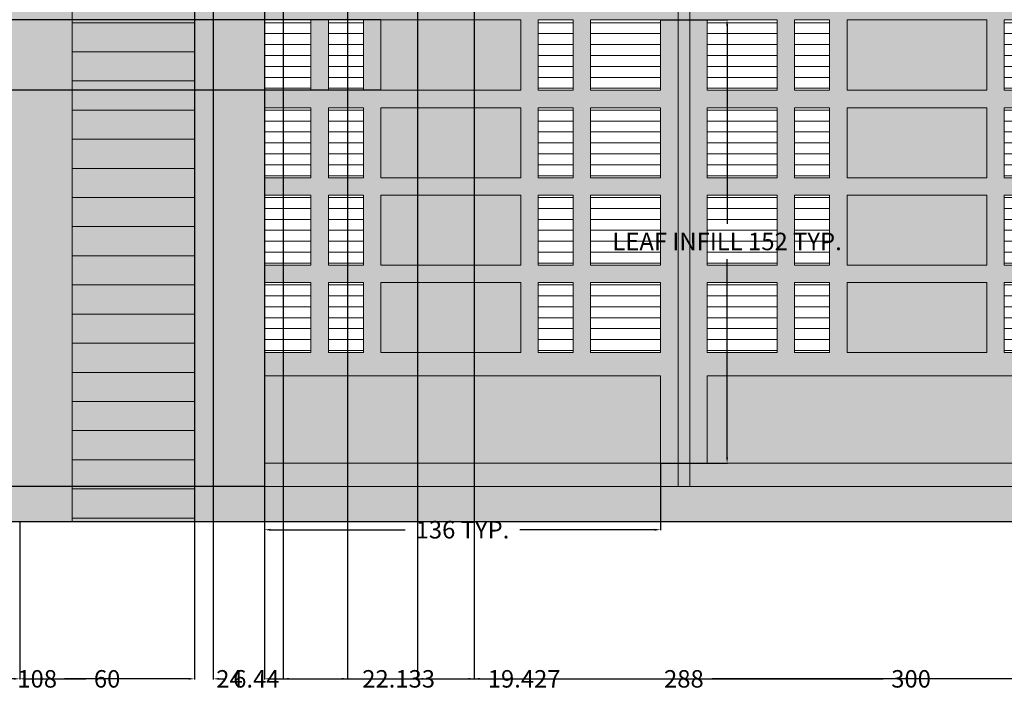
# Model space of a CAD drawing. Units: inches. Extents: x 180 to 1069, y 71 to 1267.
# Tile 2 of 8: x 546 to 884, y 71 to 301. Entities that reach past the tile are written whole.
import ezdxf

# ---------------------------------------------------------------- set-up
doc = ezdxf.new("R2010")
doc.units = ezdxf.units.IN
doc.header["$MEASUREMENT"] = 0
for name, color, linetype, lineweight in [('A-ANNO-DIMS', 2, 'Continuous', 18), ('A-COLS', 7, 'Continuous', 25), ('A-DOOR-GATE', 7, 'Continuous', 18), ('A-DOOR-PANL-PATT', 25, 'Continuous', 13), ('A-WALL', 7, 'Continuous', 30), ('A-WALL-CLAD', 7, 'Continuous', 18), ('A-WALL-CLAD-JNTS-PATT', 18, 'Continuous', 13), ('A-WALL-CLAD-PATT', 26, 'Continuous', 13)]:
    doc.layers.add(name, color=color, linetype=linetype, lineweight=lineweight)
for name, color, linetype, lineweight, true_color in [('A-DOOR-GATE-PATT', 18, 'Continuous', 13, 0x000000), ('A-DOOR-HARD-PATT', 8, 'Continuous', 13, 0x7f7f6c), ('A-DOOR-SHUT-PATT', 254, 'Continuous', 13, 0xb7d9eb), ('A-ELEV-FRAM-PATT', 53, 'Continuous', 13, 0xefd648)]:
    doc.layers.add(name, color=color, linetype=linetype, lineweight=lineweight, true_color=true_color)
doc.styles.get("Standard").update_dxf_attribs({"font": 'arial.ttf'})
doc.dimstyles.get("Standard").update_dxf_attribs({"dimtxt": 6, "dimasz": 2, "dimexe": 0.18, "dimexo": 0.0625, "dimgap": 3, "dimtad": 0, "dimtih": 1, "dimtoh": 1, "dimdec": 0, "dimzin": 0, "dimdsep": 46, "dimlunit": 3, "dimtxsty": 'Standard', "dimcen": 0.09, "dimadec": 0, "dimazin": 0, "dimtfac": 1, "dimtdec": 0, "dimtofl": 0, "dimtmove": 0, "dimatfit": 3, "dimfxl": 1, "dimtolj": 1, "dimtzin": 0, "dimarcsym": 0})

# ---------------------------------------------------------------- blocks, each defined once
blk = doc.blocks.new('GATE-LEAF-LOWER-INFILL')
for p, q in [((0, 152.23), (16, 152.23)), ((16, 152.23), (16, 128)), ((22, 152.23), (34, 152.23)), ((22, 152.23), (22, 128)), ((34, 152.23), (34, 128)), ((40, 152.23), (88, 152.23)), ((40, 152.23), (40, 128)), ((88, 152.23), (88, 128)), ((94, 152.23), (106, 152.23)), ((94, 152.23), (94, 128)), ((106, 152.23), (106, 128)), ((112, 152.23), (136, 152.23)), ((112, 152.23), (112, 128)), ((136, 152.23), (136, 128)), ((0, 128), (16, 128)), ((22, 128), (34, 128)), ((40, 128), (88, 128)), ((94, 128), (106, 128)), ((112, 128), (136, 128)), ((0, 122), (16, 122)), ((16, 122), (16, 98)), ((22, 122), (34, 122)), ((22, 122), (22, 98)), ((34, 122), (34, 98)), ((40, 122), (88, 122)), ((40, 122), (40, 98)), ((88, 122), (88, 98)), ((94, 122), (106, 122)), ((94, 122), (94, 98)), ((106, 122), (106, 98)), ((112, 122), (136, 122)), ((112, 122), (112, 98)), ((136, 122), (136, 98)), ((0, 98), (16, 98)), ((22, 98), (34, 98)), ((40, 98), (88, 98)), ((94, 98), (106, 98)), ((112, 98), (136, 98)), ((0, 92), (16, 92)), ((16, 92), (16, 68)), ((22, 92), (34, 92)), ((22, 92), (22, 68)), ((34, 92), (34, 68)), ((40, 92), (88, 92)), ((40, 92), (40, 68)), ((88, 92), (88, 68)), ((94, 92), (106, 92)), ((94, 92), (94, 68)), ((106, 92), (106, 68)), ((112, 92), (136, 92)), ((112, 92), (112, 68)), ((136, 92), (136, 68)), ((0, 68), (16, 68)), ((22, 68), (34, 68)), ((40, 68), (88, 68)), ((94, 68), (106, 68)), ((112, 68), (136, 68)), ((0, 62), (16, 62)), ((16, 62), (16, 38)), ((22, 62), (34, 62)), ((22, 62), (22, 38)), ((34, 62), (34, 38)), ((40, 62), (88, 62)), ((40, 62), (40, 38)), ((88, 62), (88, 38)), ((94, 62), (106, 62)), ((94, 62), (94, 38)), ((106, 62), (106, 38)), ((112, 62), (136, 62)), ((112, 62), (112, 38)), ((136, 62), (136, 38)), ((0, 38), (16, 38)), ((22, 38), (34, 38)), ((40, 38), (88, 38)), ((94, 38), (106, 38)), ((112, 38), (136, 38)), ((0, 30), (136, 30)), ((136, 30), (136, 0)), ((0, 0), (136, 0))]:
    blk.add_line(p, q)
blk = doc.blocks.new('*D14')
at = {"layer": 'A-ANNO-DIMS', "color": 0, "lineweight": -2, "transparency": 16777216}
for p, q in [((766.15, 301.05), (789.1, 301.05)), ((788.92, 299.05), (788.92, 231)), ((788.92, 150.82), (788.92, 218.87)), ((766.15, 148.82), (789.1, 148.82))]:
    blk.add_line(p, q, dxfattribs=at)
at = {"layer": 'A-ANNO-DIMS', "color": 0, "transparency": 16777216}
for points in [[(788.59, 299.05), (789.26, 299.05), (788.92, 301.05)], [(788.59, 150.82), (789.26, 150.82), (788.92, 148.82)]]:
    blk.add_solid(points, dxfattribs=at)
at = {"layer": 'Defpoints', "color": 0, "transparency": 16777216}
for p in [(766.09, 301.05), (788.92, 301.05), (766.09, 148.82)]:
    blk.add_point(p, dxfattribs=at)
at = {"layer": 'A-ANNO-DIMS', "color": 0, "transparency": 16777216, "insert": (788.92, 224.93), "char_height": 6, "attachment_point": 5}
blk.add_mtext('\\A1;LEAF INFILL 152 TYP.', dxfattribs=at)
blk = doc.blocks.new('*D15')
at = {"layer": 'A-ANNO-DIMS', "color": 0, "lineweight": -2, "transparency": 16777216}
for p, q in [((630.09, 148.75), (630.09, 125.8)), ((766.09, 148.75), (766.09, 125.8)), ((632.09, 125.98), (678.44, 125.98)), ((764.09, 125.98), (717.74, 125.98))]:
    blk.add_line(p, q, dxfattribs=at)
at = {"layer": 'A-ANNO-DIMS', "color": 0, "transparency": 16777216}
for points in [[(632.09, 126.31), (632.09, 125.65), (630.09, 125.98)], [(764.09, 126.31), (764.09, 125.65), (766.09, 125.98)]]:
    blk.add_solid(points, dxfattribs=at)
at = {"layer": 'Defpoints', "color": 0, "transparency": 16777216}
for p in [(630.09, 148.82), (766.09, 148.82), (766.09, 125.98)]:
    blk.add_point(p, dxfattribs=at)
at = {"layer": 'A-ANNO-DIMS', "color": 0, "transparency": 16777216, "insert": (698.09, 125.98), "char_height": 6, "attachment_point": 5}
blk.add_mtext('\\A1;136 TYP.', dxfattribs=at)
blk = doc.blocks.new('*D29')
at = {"layer": 'A-ANNO-DIMS', "color": 0, "lineweight": -2, "transparency": 16777216}
for p, q in [((306.09, 128.75), (306.09, 74.62)), ((546.09, 128.75), (546.09, 74.62)), ((308.09, 74.8), (416.42, 74.8)), ((544.09, 74.8), (435.76, 74.8))]:
    blk.add_line(p, q, dxfattribs=at)
at = {"layer": 'A-ANNO-DIMS', "color": 0, "transparency": 16777216}
for points in [[(308.09, 75.14), (308.09, 74.47), (306.09, 74.8)], [(544.09, 75.14), (544.09, 74.47), (546.09, 74.8)]]:
    blk.add_solid(points, dxfattribs=at)
at = {"layer": 'Defpoints', "color": 0, "transparency": 16777216}
for p in [(306.09, 128.82), (546.09, 128.82), (546.09, 74.8)]:
    blk.add_point(p, dxfattribs=at)
at = {"layer": 'A-ANNO-DIMS', "color": 0, "transparency": 16777216, "insert": (426.09, 74.8), "char_height": 6, "attachment_point": 5}
blk.add_mtext('\\A1;240', dxfattribs=at)
blk = doc.blocks.new('*D30')
at = {"layer": 'A-ANNO-DIMS', "color": 0, "lineweight": -2, "transparency": 16777216}
for p, q in [((546.09, 128.75), (546.09, 74.62)), ((606.09, 128.75), (606.09, 74.62)), ((548.09, 74.8), (568.78, 74.8)), ((604.09, 74.8), (583.39, 74.8))]:
    blk.add_line(p, q, dxfattribs=at)
at = {"layer": 'A-ANNO-DIMS', "color": 0, "transparency": 16777216}
for points in [[(548.09, 75.14), (548.09, 74.47), (546.09, 74.8)], [(604.09, 75.14), (604.09, 74.47), (606.09, 74.8)]]:
    blk.add_solid(points, dxfattribs=at)
at = {"layer": 'Defpoints', "color": 0, "transparency": 16777216}
for p in [(546.09, 128.82), (606.09, 128.82), (606.09, 74.8)]:
    blk.add_point(p, dxfattribs=at)
at = {"layer": 'A-ANNO-DIMS', "color": 0, "transparency": 16777216, "insert": (576.09, 74.8), "char_height": 6, "attachment_point": 5}
blk.add_mtext('\\A1;60', dxfattribs=at)
blk = doc.blocks.new('*D31')
at = {"layer": 'A-ANNO-DIMS', "color": 0, "lineweight": -2, "transparency": 16777216}
for p, q in [((546.15, 416.82), (1056.28, 416.82)), ((1056.1, 414.82), (1056.1, 278.88)), ((1056.1, 130.82), (1056.1, 266.75)), ((546.15, 128.82), (1056.28, 128.82))]:
    blk.add_line(p, q, dxfattribs=at)
at = {"layer": 'A-ANNO-DIMS', "color": 0, "transparency": 16777216}
for points in [[(1055.77, 414.82), (1056.43, 414.82), (1056.1, 416.82)], [(1055.77, 130.82), (1056.43, 130.82), (1056.1, 128.82)]]:
    blk.add_solid(points, dxfattribs=at)
at = {"layer": 'Defpoints', "color": 0, "transparency": 16777216}
for p in [(546.09, 416.82), (1056.1, 416.82), (546.09, 128.82)]:
    blk.add_point(p, dxfattribs=at)
at = {"layer": 'A-ANNO-DIMS', "color": 0, "transparency": 16777216, "insert": (1056.1, 272.82), "char_height": 6, "attachment_point": 5}
blk.add_mtext('\\A1;288', dxfattribs=at)
blk = doc.blocks.new('*D33')
at = {"layer": 'A-ANNO-DIMS', "color": 0, "lineweight": -2, "transparency": 16777216}
for p, q in [((606.09, 128.75), (606.09, 74.62)), ((630.09, 128.75), (630.09, 74.62)), ((604.09, 74.8), (602.09, 74.8)), ((632.09, 74.8), (634.09, 74.8))]:
    blk.add_line(p, q, dxfattribs=at)
at = {"layer": 'A-ANNO-DIMS', "color": 0, "transparency": 16777216}
for points in [[(604.09, 75.14), (604.09, 74.47), (606.09, 74.8)], [(632.09, 75.14), (632.09, 74.47), (630.09, 74.8)]]:
    blk.add_solid(points, dxfattribs=at)
at = {"layer": 'Defpoints', "color": 0, "transparency": 16777216}
for p in [(606.09, 128.82), (630.09, 128.82), (630.09, 74.8)]:
    blk.add_point(p, dxfattribs=at)
at = {"layer": 'A-ANNO-DIMS', "color": 0, "transparency": 16777216, "insert": (618.09, 74.8), "char_height": 6, "attachment_point": 5}
blk.add_mtext('\\A1;24', dxfattribs=at)
blk = doc.blocks.new('*D34')
at = {"layer": 'A-ANNO-DIMS', "color": 0, "lineweight": -2, "transparency": 16777216}
for p, q in [((630.09, 128.75), (630.09, 74.62)), ((918.09, 128.75), (918.09, 74.62)), ((632.09, 74.8), (764.4, 74.8)), ((916.09, 74.8), (783.77, 74.8))]:
    blk.add_line(p, q, dxfattribs=at)
at = {"layer": 'A-ANNO-DIMS', "color": 0, "transparency": 16777216}
for points in [[(632.09, 75.14), (632.09, 74.47), (630.09, 74.8)], [(916.09, 75.14), (916.09, 74.47), (918.09, 74.8)]]:
    blk.add_solid(points, dxfattribs=at)
at = {"layer": 'Defpoints', "color": 0, "transparency": 16777216}
for p in [(630.09, 128.82), (918.09, 128.82), (918.09, 74.8)]:
    blk.add_point(p, dxfattribs=at)
at = {"layer": 'A-ANNO-DIMS', "color": 0, "transparency": 16777216, "insert": (774.09, 74.8), "char_height": 6, "attachment_point": 5}
blk.add_mtext('\\A1;288', dxfattribs=at)
blk = doc.blocks.new('*D39')
at = {"layer": 'A-ANNO-DIMS', "color": 0, "lineweight": -2, "transparency": 16777216}
for p, q in [((630.02, 346.05), (191.89, 346.05)), ((192.07, 344.05), (192.07, 249.5)), ((192.07, 142.82), (192.07, 237.37)), ((630.02, 140.82), (191.89, 140.82))]:
    blk.add_line(p, q, dxfattribs=at)
at = {"layer": 'A-ANNO-DIMS', "color": 0, "transparency": 16777216}
for points in [[(191.74, 344.05), (192.41, 344.05), (192.07, 346.05)], [(191.74, 142.82), (192.41, 142.82), (192.07, 140.82)]]:
    blk.add_solid(points, dxfattribs=at)
at = {"layer": 'Defpoints', "color": 0, "transparency": 16777216}
for p in [(192.07, 346.05), (630.09, 346.05), (630.09, 140.82)]:
    blk.add_point(p, dxfattribs=at)
at = {"layer": 'A-ANNO-DIMS', "color": 0, "transparency": 16777216, "insert": (192.07, 243.43), "char_height": 6, "attachment_point": 5}
blk.add_mtext('\\A1;205.23', dxfattribs=at)
blk = doc.blocks.new('*D43')
at = {"layer": 'A-ANNO-DIMS', "color": 0, "lineweight": -2, "transparency": 16777216}
for p, q in [((670.02, 301.05), (191.89, 301.05)), ((192.07, 299.05), (192.07, 295)), ((192.07, 278.82), (192.07, 282.87)), ((670.02, 276.82), (191.89, 276.82))]:
    blk.add_line(p, q, dxfattribs=at)
at = {"layer": 'A-ANNO-DIMS', "color": 0, "transparency": 16777216}
for points in [[(191.74, 299.05), (192.41, 299.05), (192.07, 301.05)], [(191.74, 278.82), (192.41, 278.82), (192.07, 276.82)]]:
    blk.add_solid(points, dxfattribs=at)
at = {"layer": 'Defpoints', "color": 0, "transparency": 16777216}
for p in [(670.09, 301.05), (192.07, 276.82), (670.09, 276.82)]:
    blk.add_point(p, dxfattribs=at)
at = {"layer": 'A-ANNO-DIMS', "color": 0, "transparency": 16777216, "insert": (192.07, 288.93), "char_height": 6, "attachment_point": 5}
blk.add_mtext('\\A1;24.23', dxfattribs=at)
blk = doc.blocks.new('*D58')
at = {"layer": 'A-ANNO-DIMS', "color": 0, "lineweight": -2, "transparency": 16777216}
for p, q in [((606.09, 1010.75), (606.09, 74.62)), ((498.09, 956.75), (498.09, 74.62)), ((500.09, 74.8), (542.74, 74.8)), ((604.09, 74.8), (561.44, 74.8))]:
    blk.add_line(p, q, dxfattribs=at)
at = {"layer": 'A-ANNO-DIMS', "color": 0, "transparency": 16777216}
for points in [[(500.09, 75.14), (500.09, 74.47), (498.09, 74.8)], [(604.09, 75.14), (604.09, 74.47), (606.09, 74.8)]]:
    blk.add_solid(points, dxfattribs=at)
at = {"layer": 'Defpoints', "color": 0, "transparency": 16777216}
for p in [(606.09, 1010.82), (498.09, 956.82), (606.09, 74.8)]:
    blk.add_point(p, dxfattribs=at)
at = {"layer": 'A-ANNO-DIMS', "color": 0, "transparency": 16777216, "insert": (552.09, 74.8), "char_height": 6, "attachment_point": 5}
blk.add_mtext('\\A1;108', dxfattribs=at)
blk = doc.blocks.new('*D65')
at = {"layer": 'A-ANNO-DIMS', "color": 0, "lineweight": -2, "transparency": 16777216}
for p, q in [((636.53, 557.75), (636.53, 74.62)), ((658.66, 557.75), (658.66, 74.62)), ((638.53, 74.8), (656.66, 74.8)), ((658.66, 74.8), (660.66, 74.8))]:
    blk.add_line(p, q, dxfattribs=at)
at = {"layer": 'A-ANNO-DIMS', "color": 0, "transparency": 16777216}
for points in [[(638.53, 75.14), (638.53, 74.47), (636.53, 74.8)], [(656.66, 75.14), (656.66, 74.47), (658.66, 74.8)]]:
    blk.add_solid(points, dxfattribs=at)
at = {"layer": 'Defpoints', "color": 0, "transparency": 16777216}
for p in [(636.53, 557.82), (658.66, 557.82), (658.66, 74.8)]:
    blk.add_point(p, dxfattribs=at)
at = {"layer": 'A-ANNO-DIMS', "color": 0, "transparency": 16777216, "insert": (676.17, 74.8), "char_height": 6, "attachment_point": 5}
blk.add_mtext('\\A1;22.133', dxfattribs=at)
blk = doc.blocks.new('*D66')
at = {"layer": 'A-ANNO-DIMS', "color": 0, "lineweight": -2, "transparency": 16777216}
for p, q in [((606.09, 647.75), (606.09, 74.62)), ((612.53, 557.75), (612.53, 74.62)), ((604.09, 74.8), (602.09, 74.8)), ((614.53, 74.8), (616.53, 74.8))]:
    blk.add_line(p, q, dxfattribs=at)
at = {"layer": 'A-ANNO-DIMS', "color": 0, "transparency": 16777216}
for points in [[(604.09, 75.14), (604.09, 74.47), (606.09, 74.8)], [(614.53, 75.14), (614.53, 74.47), (612.53, 74.8)]]:
    blk.add_solid(points, dxfattribs=at)
at = {"layer": 'Defpoints', "color": 0, "transparency": 16777216}
for p in [(606.09, 647.82), (612.53, 557.82), (612.53, 74.8)]:
    blk.add_point(p, dxfattribs=at)
at = {"layer": 'A-ANNO-DIMS', "color": 0, "transparency": 16777216, "insert": (627.32, 74.8), "char_height": 6, "attachment_point": 5}
blk.add_mtext('\\A1;6.44', dxfattribs=at)
blk = doc.blocks.new('*D67')
at = {"layer": 'A-ANNO-DIMS', "color": 0, "lineweight": -2, "transparency": 16777216}
for p, q in [((682.66, 557.75), (682.66, 74.62)), ((702.09, 557.75), (702.09, 74.62)), ((684.66, 74.8), (700.09, 74.8)), ((702.09, 74.8), (704.09, 74.8))]:
    blk.add_line(p, q, dxfattribs=at)
at = {"layer": 'A-ANNO-DIMS', "color": 0, "transparency": 16777216}
for points in [[(684.66, 75.14), (684.66, 74.47), (682.66, 74.8)], [(700.09, 75.14), (700.09, 74.47), (702.09, 74.8)]]:
    blk.add_solid(points, dxfattribs=at)
at = {"layer": 'Defpoints', "color": 0, "transparency": 16777216}
for p in [(682.66, 557.82), (702.09, 557.82), (702.09, 74.8)]:
    blk.add_point(p, dxfattribs=at)
at = {"layer": 'A-ANNO-DIMS', "color": 0, "transparency": 16777216, "insert": (719.26, 74.8), "char_height": 6, "attachment_point": 5}
blk.add_mtext('\\A1;19.427', dxfattribs=at)
blk = doc.blocks.new('*D68')
at = {"layer": 'A-ANNO-DIMS', "color": 0, "lineweight": -2, "transparency": 16777216}
for p, q in [((702.09, 557.75), (702.09, 74.62)), ((1002.09, 557.75), (1002.09, 74.62)), ((704.09, 74.8), (842.47, 74.8)), ((1000.09, 74.8), (861.7, 74.8))]:
    blk.add_line(p, q, dxfattribs=at)
at = {"layer": 'A-ANNO-DIMS', "color": 0, "transparency": 16777216}
for points in [[(704.09, 75.14), (704.09, 74.47), (702.09, 74.8)], [(1000.09, 75.14), (1000.09, 74.47), (1002.09, 74.8)]]:
    blk.add_solid(points, dxfattribs=at)
at = {"layer": 'Defpoints', "color": 0, "transparency": 16777216}
for p in [(702.09, 557.82), (1002.09, 557.82), (1002.09, 74.8)]:
    blk.add_point(p, dxfattribs=at)
at = {"layer": 'A-ANNO-DIMS', "color": 0, "transparency": 16777216, "insert": (852.09, 74.8), "char_height": 6, "attachment_point": 5}
blk.add_mtext('\\A1;300', dxfattribs=at)

msp = doc.modelspace()

# ---------------------------------------------------------------- hatches: boundary and pattern name
at = {"layer": 'A-DOOR-GATE-PATT'}
h = msp.add_hatch(color=256, dxfattribs=at)
h.dxf.hatch_style = 1
h.paths.add_polyline_path([(772.0875, 346.0477), (630.0875, 346.0477), (630.0875, 338.0477), (646.0875, 338.0477), (646.0875, 307.0477), (630.0875, 307.0477), (630.0875, 301.0477), (646.0875, 301.0477), (646.0875, 276.8159), (630.0875, 276.8159), (630.0875, 270.8159), (646.0875, 270.8159), (646.0875, 246.8159), (630.0875, 246.8159), (630.0875, 240.8159), (646.0875, 240.8159), (646.0875, 216.8159), (630.0875, 216.8159), (630.0875, 210.8159), (646.0875, 210.8159), (646.0875, 186.8159), (630.0875, 186.8159), (630.0875, 178.8159), (766.0875, 178.8159), (766.0875, 148.8159), (630.0875, 148.8159), (630.0875, 140.8159), (772.0875, 140.8159)])
h.paths.add_polyline_path([(670.0875, 338.0477), (718.0875, 338.0477), (718.0875, 307.0477), (670.0875, 307.0477)], flags=16)
h.paths.add_polyline_path([(664.0875, 338.0477), (664.0875, 307.0477), (652.0875, 307.0477), (652.0875, 338.0477)], flags=16)
h.paths.add_polyline_path([(670.0875, 301.0477), (718.0875, 301.0477), (718.0875, 276.8159), (670.0875, 276.8159)], flags=16)
h.paths.add_polyline_path([(664.0875, 301.0477), (664.0875, 276.8159), (652.0875, 276.8159), (652.0875, 301.0477)], flags=16)
h.paths.add_polyline_path([(724.0875, 338.0477), (736.0875, 338.0477), (736.0875, 307.0477), (724.0875, 307.0477)], flags=16)
h.paths.add_polyline_path([(724.0875, 301.0477), (736.0875, 301.0477), (736.0875, 276.8159), (724.0875, 276.8159)], flags=16)
h.paths.add_polyline_path([(670.0875, 270.8159), (718.0875, 270.8159), (718.0875, 246.8159), (670.0875, 246.8159)], flags=16)
h.paths.add_polyline_path([(664.0875, 270.8159), (664.0875, 246.8159), (652.0875, 246.8159), (652.0875, 270.8159)], flags=16)
h.paths.add_polyline_path([(742.0875, 338.0477), (766.0875, 338.0477), (766.0875, 307.0477), (742.0875, 307.0477)], flags=16)
h.paths.add_polyline_path([(742.0875, 301.0477), (766.0875, 301.0477), (766.0875, 276.8159), (742.0875, 276.8159)], flags=16)
h.paths.add_polyline_path([(724.0875, 270.8159), (736.0875, 270.8159), (736.0875, 246.8159), (724.0875, 246.8159)], flags=16)
h.paths.add_polyline_path([(670.0875, 240.8159), (718.0875, 240.8159), (718.0875, 216.8159), (670.0875, 216.8159)], flags=16)
h.paths.add_polyline_path([(664.0875, 240.8159), (664.0875, 216.8159), (652.0875, 216.8159), (652.0875, 240.8159)], flags=16)
h.paths.add_polyline_path([(742.0875, 270.8159), (766.0875, 270.8159), (766.0875, 246.8159), (742.0875, 246.8159)], flags=16)
h.paths.add_polyline_path([(724.0875, 240.8159), (736.0875, 240.8159), (736.0875, 216.8159), (724.0875, 216.8159)], flags=16)
h.paths.add_polyline_path([(742.0875, 240.8159), (766.0875, 240.8159), (766.0875, 216.8159), (742.0875, 216.8159)], flags=16)
h.paths.add_polyline_path([(670.0875, 210.8159), (718.0875, 210.8159), (718.0875, 186.8159), (670.0875, 186.8159)], flags=16)
h.paths.add_polyline_path([(664.0875, 210.8159), (664.0875, 186.8159), (652.0875, 186.8159), (652.0875, 210.8159)], flags=16)
h.paths.add_polyline_path([(724.0875, 210.8159), (736.0875, 210.8159), (736.0875, 186.8159), (724.0875, 186.8159)], flags=16)
h.paths.add_polyline_path([(742.0875, 210.8159), (766.0875, 210.8159), (766.0875, 186.8159), (742.0875, 186.8159)], flags=16)
h.paths.add_polyline_path([(918.0875, 346.0477), (776.0875, 346.0477), (776.0875, 140.8159), (918.0875, 140.8159), (918.0875, 148.8159), (782.0875, 148.8159), (782.0875, 178.8159), (918.0875, 178.8159), (918.0875, 186.8159), (902.0875, 186.8159), (902.0875, 210.8159), (918.0875, 210.8159), (918.0875, 216.8159), (902.0875, 216.8159), (902.0875, 240.8159), (918.0875, 240.8159), (918.0875, 246.8159), (902.0875, 246.8159), (902.0875, 270.8159), (918.0875, 270.8159), (918.0875, 276.8159), (902.0875, 276.8159), (902.0875, 301.0477), (918.0875, 301.0477), (918.0875, 307.0477), (902.0875, 307.0477), (902.0875, 338.0477), (918.0875, 338.0477)])
h.paths.add_polyline_path([(782.0875, 338.0477), (806.0875, 338.0477), (806.0875, 307.0477), (782.0875, 307.0477)], flags=16)
h.paths.add_polyline_path([(812.0875, 338.0477), (824.0875, 338.0477), (824.0875, 307.0477), (812.0875, 307.0477)], flags=16)
h.paths.add_polyline_path([(782.0875, 301.0477), (806.0875, 301.0477), (806.0875, 276.8159), (782.0875, 276.8159)], flags=16)
h.paths.add_polyline_path([(830.0875, 338.0477), (878.0875, 338.0477), (878.0875, 307.0477), (830.0875, 307.0477)], flags=16)
h.paths.add_polyline_path([(812.0875, 301.0477), (824.0875, 301.0477), (824.0875, 276.8159), (812.0875, 276.8159)], flags=16)
h.paths.add_polyline_path([(830.0875, 301.0477), (878.0875, 301.0477), (878.0875, 276.8159), (830.0875, 276.8159)], flags=16)
h.paths.add_polyline_path([(782.0875, 270.8159), (806.0875, 270.8159), (806.0875, 246.8159), (782.0875, 246.8159)], flags=16)
h.paths.add_polyline_path([(812.0875, 270.8159), (824.0875, 270.8159), (824.0875, 246.8159), (812.0875, 246.8159)], flags=16)
h.paths.add_polyline_path([(830.0875, 270.8159), (878.0875, 270.8159), (878.0875, 246.8159), (830.0875, 246.8159)], flags=16)
h.paths.add_polyline_path([(782.0875, 240.8159), (806.0875, 240.8159), (806.0875, 216.8159), (782.0875, 216.8159)], flags=16)
h.paths.add_polyline_path([(884.0875, 338.0477), (896.0875, 338.0477), (896.0875, 307.0477), (884.0875, 307.0477)], flags=16)
h.paths.add_polyline_path([(812.0875, 240.8159), (824.0875, 240.8159), (824.0875, 216.8159), (812.0875, 216.8159)], flags=16)
h.paths.add_polyline_path([(884.0875, 301.0477), (896.0875, 301.0477), (896.0875, 276.8159), (884.0875, 276.8159)], flags=16)
h.paths.add_polyline_path([(830.0875, 240.8159), (878.0875, 240.8159), (878.0875, 216.8159), (830.0875, 216.8159)], flags=16)
h.paths.add_polyline_path([(884.0875, 270.8159), (896.0875, 270.8159), (896.0875, 246.8159), (884.0875, 246.8159)], flags=16)
h.paths.add_polyline_path([(782.0875, 210.8159), (806.0875, 210.8159), (806.0875, 186.8159), (782.0875, 186.8159)], flags=16)
h.paths.add_polyline_path([(812.0875, 210.8159), (824.0875, 210.8159), (824.0875, 186.8159), (812.0875, 186.8159)], flags=16)
h.paths.add_polyline_path([(830.0875, 210.8159), (878.0875, 210.8159), (878.0875, 186.8159), (830.0875, 186.8159)], flags=16)
h.paths.add_polyline_path([(884.0875, 240.8159), (896.0875, 240.8159), (896.0875, 216.8159), (884.0875, 216.8159)], flags=16)
h.paths.add_polyline_path([(884.0875, 210.8159), (896.0875, 210.8159), (896.0875, 186.8159), (884.0875, 186.8159)], flags=16)
h = msp.add_hatch(dxfattribs=at)
h.set_pattern_fill('ANSI31', color=256, scale=30, angle=135)
h.paths.add_polyline_path([(646.0875, 338.0477), (630.0875, 338.0477), (630.0875, 307.0477), (646.0875, 307.0477)])
h.paths.add_polyline_path([(646.0875, 301.0477), (630.0875, 301.0477), (630.0875, 276.8159), (646.0875, 276.8159)])
h.paths.add_polyline_path([(664.0875, 301.0477), (652.0875, 301.0477), (652.0875, 276.8159), (664.0875, 276.8159)])
h.paths.add_polyline_path([(664.0875, 270.8159), (652.0875, 270.8159), (652.0875, 246.8159), (664.0875, 246.8159)])
h.paths.add_polyline_path([(646.0875, 270.8159), (630.0875, 270.8159), (630.0875, 246.8159), (646.0875, 246.8159)])
h.paths.add_polyline_path([(646.0875, 240.8159), (630.0875, 240.8159), (630.0875, 216.8159), (646.0875, 216.8159)])
h.paths.add_polyline_path([(664.0875, 240.8159), (652.0875, 240.8159), (652.0875, 216.8159), (664.0875, 216.8159)])
h.paths.add_polyline_path([(664.0875, 210.8159), (652.0875, 210.8159), (652.0875, 186.8159), (664.0875, 186.8159)])
h.paths.add_polyline_path([(646.0875, 210.8159), (630.0875, 210.8159), (630.0875, 186.8159), (646.0875, 186.8159)])
h.paths.add_polyline_path([(736.0875, 301.0477), (724.0875, 301.0477), (724.0875, 276.8159), (736.0875, 276.8159)])
h.paths.add_polyline_path([(766.0875, 301.0477), (742.0875, 301.0477), (742.0875, 276.8159), (766.0875, 276.8159)])
h.paths.add_polyline_path([(766.0875, 270.8159), (742.0875, 270.8159), (742.0875, 246.8159), (766.0875, 246.8159)])
h.paths.add_polyline_path([(766.0875, 338.0477), (742.0875, 338.0477), (742.0875, 307.0477), (766.0875, 307.0477)])
h.paths.add_polyline_path([(736.0875, 270.8159), (724.0875, 270.8159), (724.0875, 246.8159), (736.0875, 246.8159)])
h.paths.add_polyline_path([(736.0875, 240.8159), (724.0875, 240.8159), (724.0875, 216.8159), (736.0875, 216.8159)])
h.paths.add_polyline_path([(766.0875, 240.8159), (742.0875, 240.8159), (742.0875, 216.8159), (766.0875, 216.8159)])
h.paths.add_polyline_path([(766.0875, 210.8159), (742.0875, 210.8159), (742.0875, 186.8159), (766.0875, 186.8159)])
h.paths.add_polyline_path([(736.0875, 210.8159), (724.0875, 210.8159), (724.0875, 186.8159), (736.0875, 186.8159)])
h.paths.add_polyline_path([(806.0875, 210.8159), (782.0875, 210.8159), (782.0875, 186.8159), (806.0875, 186.8159)])
h.paths.add_polyline_path([(806.0875, 240.8159), (782.0875, 240.8159), (782.0875, 216.8159), (806.0875, 216.8159)])
h.paths.add_polyline_path([(806.0875, 270.8159), (782.0875, 270.8159), (782.0875, 246.8159), (806.0875, 246.8159)])
h.paths.add_polyline_path([(806.0875, 301.0477), (782.0875, 301.0477), (782.0875, 276.8159), (806.0875, 276.8159)])
h.paths.add_polyline_path([(806.0875, 338.0477), (782.0875, 338.0477), (782.0875, 307.0477), (806.0875, 307.0477)])
h.paths.add_polyline_path([(824.0875, 301.0477), (812.0875, 301.0477), (812.0875, 276.8159), (824.0875, 276.8159)])
h.paths.add_polyline_path([(824.0875, 270.8159), (812.0875, 270.8159), (812.0875, 246.8159), (824.0875, 246.8159)])
h.paths.add_polyline_path([(824.0875, 240.8159), (812.0875, 240.8159), (812.0875, 216.8159), (824.0875, 216.8159)])
h.paths.add_polyline_path([(824.0875, 210.8159), (812.0875, 210.8159), (812.0875, 186.8159), (824.0875, 186.8159)])
h.paths.add_polyline_path([(918.0875, 338.0477), (902.0875, 338.0477), (902.0875, 307.0477), (918.0875, 307.0477)])
h.paths.add_polyline_path([(918.0875, 301.0477), (902.0875, 301.0477), (902.0875, 276.8159), (918.0875, 276.8159)])
h.paths.add_polyline_path([(918.0875, 270.8159), (902.0875, 270.8159), (902.0875, 246.8159), (918.0875, 246.8159)])
h.paths.add_polyline_path([(918.0875, 240.8159), (902.0875, 240.8159), (902.0875, 216.8159), (918.0875, 216.8159)])
h.paths.add_polyline_path([(918.0875, 210.8159), (902.0875, 210.8159), (902.0875, 186.8159), (918.0875, 186.8159)])
h.paths.add_polyline_path([(896.0875, 210.8159), (884.0875, 210.8159), (884.0875, 186.8159), (896.0875, 186.8159)])
h.paths.add_polyline_path([(896.0875, 240.8159), (884.0875, 240.8159), (884.0875, 216.8159), (896.0875, 216.8159)])
h.paths.add_polyline_path([(896.0875, 270.8159), (884.0875, 270.8159), (884.0875, 246.8159), (896.0875, 246.8159)])
h.paths.add_polyline_path([(896.0875, 301.0477), (884.0875, 301.0477), (884.0875, 276.8159), (896.0875, 276.8159)])
at = {"layer": 'A-DOOR-HARD-PATT'}
h = msp.add_hatch(color=256, dxfattribs=at)
h.dxf.hatch_style = 1
h.paths.add_polyline_path([(776.0875, 346.0477), (772.0875, 346.0477), (772.0875, 140.8159), (776.0875, 140.8159)])
h = msp.add_hatch(color=256, dxfattribs=at)
h.dxf.hatch_style = 1
h.paths.add_polyline_path([(918.0875, 140.8159), (776.0875, 140.8159), (772.0875, 140.8159), (630.0875, 140.8159), (630.0875, 128.8159), (918.0875, 128.8159)])
at = {"layer": 'A-DOOR-PANL-PATT'}
h = msp.add_hatch(color=256, dxfattribs=at)
h.dxf.hatch_style = 1
h.paths.add_polyline_path([(766.0875, 178.8159), (630.0875, 178.8159), (630.0875, 148.8159), (766.0875, 148.8159)])
h.paths.add_polyline_path([(918.0875, 178.8159), (782.0875, 178.8159), (782.0875, 148.8159), (918.0875, 148.8159)])
h.paths.add_polyline_path([(878.0875, 210.8159), (830.0875, 210.8159), (830.0875, 186.8159), (878.0875, 186.8159)])
h.paths.add_polyline_path([(878.0875, 240.8159), (830.0875, 240.8159), (830.0875, 216.8159), (878.0875, 216.8159)])
h.paths.add_polyline_path([(878.0875, 270.8159), (830.0875, 270.8159), (830.0875, 246.8159), (878.0875, 246.8159)])
h.paths.add_polyline_path([(878.0875, 301.0477), (830.0875, 301.0477), (830.0875, 276.8159), (878.0875, 276.8159)])
h.paths.add_polyline_path([(718.0875, 301.0477), (670.0875, 301.0477), (670.0875, 276.8159), (718.0875, 276.8159)])
h.paths.add_polyline_path([(718.0875, 270.8159), (670.0875, 270.8159), (670.0875, 246.8159), (718.0875, 246.8159)])
h.paths.add_polyline_path([(718.0875, 240.8159), (670.0875, 240.8159), (670.0875, 216.8159), (718.0875, 216.8159)])
h.paths.add_polyline_path([(718.0875, 210.8159), (670.0875, 210.8159), (670.0875, 186.8159), (718.0875, 186.8159)])
at = {"layer": 'A-DOOR-SHUT-PATT'}
h = msp.add_hatch(color=256, dxfattribs=at)
h.dxf.hatch_style = 1
h.paths.add_polyline_path([(546.0875, 416.8159), (306.0875, 416.8159), (306.0875, 140.8159), (546.0875, 140.8159)])
h.paths.add_polyline_path([(306.0875, 416.8159), (288.0875, 416.8159), (288.0875, 128.8159), (306.0875, 128.8159)])
h.paths.add_polyline_path([(546.0875, 140.8159), (306.0875, 140.8159), (306.0875, 128.8159), (546.0875, 128.8159)])
h.paths.add_polyline_path([(564.0875, 416.8159), (546.0875, 416.8159), (546.0875, 140.8159), (546.0875, 128.8159), (564.0875, 128.8159)])
at = {"layer": 'A-ELEV-FRAM-PATT'}
h = msp.add_hatch(color=256, dxfattribs=at)
h.dxf.hatch_style = 1
h.paths.add_polyline_path([(354.0875, 1184.8159), (654.0875, 1184.8159), (654.0875, 974.8159), (726.0875, 974.8159), (726.0875, 1208.8159), (288.0875, 1208.8159), (288.0875, 897.6348), (304.7188, 897.6348), (304.7188, 883.4805), (288.0875, 883.4805), (288.0875, 866.8025), (304.7188, 866.8025), (304.7188, 852.6482), (288.0875, 852.6482), (288.0875, 835.9702), (304.7188, 835.9702), (304.7188, 821.8159), (288.0875, 821.8159), (288.0875, 805.1379), (304.7188, 805.1379), (304.7188, 790.9836), (288.0875, 790.9836), (288.0875, 774.3056), (304.7188, 774.3056), (304.7188, 760.1513), (288.0875, 760.1513), (288.0875, 743.4733), (304.7188, 743.4733), (304.7188, 729.319), (288.0875, 729.319), (288.0875, 434.8159), (354.0875, 434.8159), (354.0875, 456.1177), (317.1892, 456.1177), (317.1892, 516.1177), (354.0875, 516.1177), (354.0875, 924.0304), (317.1892, 924.0304), (317.1892, 984.0304), (354.0875, 984.0304)])
h.paths.add_polyline_path([(1002.0875, 869.8159), (702.0875, 869.8159), (702.0875, 791.8159), (726.0875, 791.8159), (726.0875, 845.8159), (978.0875, 845.8159), (978.0875, 581.8159), (726.0875, 581.8159), (726.0875, 647.8159), (702.0875, 647.8159), (702.0875, 557.8159), (1002.0875, 557.8159)])
h.paths.add_polyline_path([(906.0875, 1080.2003), (882.0875, 1080.2003), (882.0875, 1056.2003), (906.0875, 1056.2003)])
h.paths.add_polyline_path([(906.0875, 996.2003), (882.0875, 996.2003), (882.0875, 972.2003), (906.0875, 972.2003)])
h.paths.add_polyline_path([(636.5273, 869.8159), (612.5273, 869.8159), (612.5273, 845.8159), (636.5273, 845.8159)], flags=17)
h.paths.add_polyline_path([(682.6602, 869.8159), (658.6602, 869.8159), (658.6602, 845.8159), (682.6602, 845.8159)], flags=17)
h.paths.add_polyline_path([(636.5273, 581.8159), (612.5273, 581.8159), (612.5273, 557.8159), (636.5273, 557.8159)], flags=17)
h.paths.add_polyline_path([(682.6602, 581.8159), (658.6602, 581.8159), (658.6602, 557.8159), (682.6602, 557.8159)], flags=17)
h.paths.add_polyline_path([(942.0875, 358.0477), (918.0875, 358.0477), (918.0875, 128.8159), (942.0875, 128.8159)])
h.paths.add_polyline_path([(630.0875, 358.0477), (606.0875, 358.0477), (606.0875, 128.8159), (630.0875, 128.8159)])
at = {"layer": 'A-WALL-CLAD-JNTS-PATT'}
h = msp.add_hatch(dxfattribs=at)
h.set_pattern_fill('ANSI31', color=256, scale=80, angle=135)
h.paths.add_polyline_path([(288.0875, 416.8159), (246.0875, 416.8159), (246.0875, 128.8159), (288.0875, 128.8159)])
h.paths.add_polyline_path([(606.0875, 358.0477), (600.0875, 358.0477), (600.0875, 370.0477), (606.0875, 370.0477), (606.0875, 416.8159), (564.0875, 416.8159), (564.0875, 128.8159), (606.0875, 128.8159)])
h.paths.add_polyline_path([(288.0875, 729.319), (262.2193, 729.319), (262.2193, 743.4733), (288.0875, 743.4733), (288.0875, 760.1513), (262.2193, 760.1513), (262.2193, 774.3056), (288.0875, 774.3056), (288.0875, 790.9836), (262.2193, 790.9836), (262.2193, 805.1379), (288.0875, 805.1379), (288.0875, 821.8159), (262.2193, 821.8159), (262.2193, 835.9702), (288.0875, 835.9702), (288.0875, 852.6482), (262.2193, 852.6482), (262.2193, 866.8025), (288.0875, 866.8025), (288.0875, 883.4805), (262.2193, 883.4805), (262.2193, 897.6348), (288.0875, 897.6348), (288.0875, 1208.8159), (246.0875, 1208.8159), (246.0875, 434.8159), (288.0875, 434.8159)])
at = {"layer": 'A-WALL-CLAD-PATT'}
h = msp.add_hatch(color=256, dxfattribs=at)
h.dxf.hatch_style = 1
h.paths.add_polyline_path([(606.0875, 358.0477), (600.0875, 358.0477), (600.0875, 370.0477), (606.0875, 370.0477), (606.0875, 416.8159), (564.0875, 416.8159), (564.0875, 128.8159), (606.0875, 128.8159)])

# ---------------------------------------------------------------- linework, layer by layer
at = {"layer": 'A-COLS'}
for p, q in [((606.0875, 358.0477), (606.0875, 128.8159)), ((630.0875, 358.0477), (630.0875, 128.8159))]:
    msp.add_line(p, q, dxfattribs=at)
at = {"layer": 'A-DOOR-GATE'}
for p, q in [((772.0875, 346.0477), (772.0875, 140.8159)), ((776.0875, 346.0477), (776.0875, 140.8159)), ((630.0875, 140.8159), (772.0875, 140.8159)), ((776.0875, 140.8159), (772.0875, 140.8159)), ((776.0875, 140.8159), (918.0875, 140.8159))]:
    msp.add_line(p, q, dxfattribs=at)
at = {"layer": 'A-WALL'}
msp.add_line((246.0875, 128.8159), (978.0875, 128.8159), dxfattribs=at)
at = {"layer": 'A-WALL-CLAD'}
msp.add_line((564.0875, 416.8159), (564.0875, 128.8159), dxfattribs=at)

# ---------------------------------------------------------------- block references
at = {"layer": 'A-DOOR-GATE'}
msp.add_blockref('GATE-LEAF-LOWER-INFILL', (630.0875, 148.8159), dxfattribs=at)
at = {"layer": 'A-DOOR-GATE', "extrusion": (0, 0, -1), "zscale": -1}
msp.add_blockref('GATE-LEAF-LOWER-INFILL', (-918.0875, 148.8159), dxfattribs=at)

# ---------------------------------------------------------------- dimensions: what is measured, and where the dimension line sits
at = {"layer": 'A-ANNO-DIMS'}
for base, p1, p2, override, picture, middle in [((606.0875, 74.8024), (498.0875, 956.8159), (606.0875, 1010.8159), {"dimdec": 0, "dimlfac": 1, "dimrnd": 0, "dimzin": 0, "dimdsep": 46, "dimlunit": 2}, '*D58', (552.0875, 74.8024)), ((612.5273, 74.8024), (606.0875, 647.8159), (612.5273, 557.8159), {"dimdec": 2, "dimlfac": 1, "dimrnd": 0, "dimzin": 0, "dimdsep": 46, "dimlunit": 2}, '*D66', (627.324, 74.8024)), ((658.6602, 74.8024), (636.5273, 557.8159), (658.6602, 557.8159), {"dimdec": 3, "dimlfac": 1, "dimrnd": 0, "dimzin": 0, "dimdsep": 46, "dimlunit": 2}, '*D65', (676.1657, 74.8024)), ((702.0875, 74.8024), (682.6602, 557.8159), (702.0875, 557.8159), {"dimdec": 3, "dimlfac": 1, "dimrnd": 0, "dimzin": 0, "dimdsep": 46, "dimlunit": 2}, '*D67', (719.2594, 74.8024)), ((1002.0875, 74.8024), (702.0875, 557.8159), (1002.0875, 557.8159), {"dimdec": 0, "dimlfac": 1, "dimrnd": 0, "dimzin": 0, "dimdsep": 46, "dimlunit": 2}, '*D68', (852.0875, 74.8024)), ((546.0875, 74.8024), (306.0875, 128.8159), (546.0875, 128.8159), {"dimdec": 0, "dimlfac": 1, "dimrnd": 0, "dimzin": 0, "dimdsep": 46, "dimlunit": 2}, '*D29', (426.0875, 74.8024)), ((606.0875, 74.8024), (546.0875, 128.8159), (606.0875, 128.8159), {"dimdec": 0, "dimlfac": 1, "dimrnd": 0, "dimzin": 0, "dimdsep": 46, "dimlunit": 2}, '*D30', (576.0875, 74.8024)), ((630.0875, 74.8024), (606.0875, 128.8159), (630.0875, 128.8159), {"dimdec": 0, "dimlfac": 1, "dimrnd": 0, "dimzin": 0, "dimdsep": 46, "dimlunit": 2}, '*D33', (618.0875, 74.8024)), ((918.0875, 74.8024), (630.0875, 128.8159), (918.0875, 128.8159), {"dimdec": 0, "dimlfac": 1, "dimrnd": 0, "dimzin": 0, "dimdsep": 46, "dimlunit": 2}, '*D34', (774.0875, 74.8024))]:
    dim = msp.add_linear_dim(base=base, p1=p1, p2=p2, dimstyle='Standard', override=override, dxfattribs=at)
    dim.commit()
    dim.dimension.update_dxf_attribs({"geometry": picture, "text_midpoint": middle})
for base, p1, p2, override, picture, middle in [((1056.101, 416.8159), (546.0875, 128.8159), (546.0875, 416.8159), {"dimdec": 0, "dimlfac": 1, "dimrnd": 0, "dimzin": 0, "dimdsep": 46, "dimlunit": 2}, '*D31', (1056.101, 272.8159)), ((192.074, 346.0477), (630.0875, 140.8159), (630.0875, 346.0477), {"dimdec": 2, "dimlfac": 1, "dimrnd": 0, "dimzin": 0, "dimdsep": 46, "dimlunit": 2}, '*D39', (192.074, 243.4318)), ((192.074, 276.8159), (670.0875, 301.0477), (670.0875, 276.8159), {"dimdec": 2, "dimlfac": 1, "dimrnd": 0, "dimzin": 0, "dimdsep": 46, "dimlunit": 2}, '*D43', (192.074, 288.9318))]:
    dim = msp.add_linear_dim(base=base, p1=p1, p2=p2, angle=90, dimstyle='Standard', override=override, dxfattribs=at)
    dim.commit()
    dim.dimension.update_dxf_attribs({"geometry": picture, "text_midpoint": middle})
dim = msp.add_linear_dim(base=(788.9222, 301.0477), p1=(766.0875, 148.8159), p2=(766.0875, 301.0477), angle=90, text='LEAF INFILL <> TYP.', dimstyle='Standard', override={"dimdec": 0, "dimlfac": 1, "dimrnd": 0, "dimzin": 0, "dimdsep": 46, "dimlunit": 2}, dxfattribs=at)
dim.commit()
dim.dimension.update_dxf_attribs({"geometry": '*D14', "text_midpoint": (788.9222, 224.9318)})
dim = msp.add_linear_dim(base=(766.0875, 125.9811), p1=(630.0875, 148.8159), p2=(766.0875, 148.8159), text='<> TYP.', dimstyle='Standard', override={"dimdec": 0, "dimlfac": 1, "dimrnd": 0, "dimzin": 0, "dimdsep": 46, "dimlunit": 2}, dxfattribs=at)
dim.commit()
dim.dimension.update_dxf_attribs({"geometry": '*D15', "text_midpoint": (698.0875, 125.9811)})

doc.saveas('drawing.dxf')
